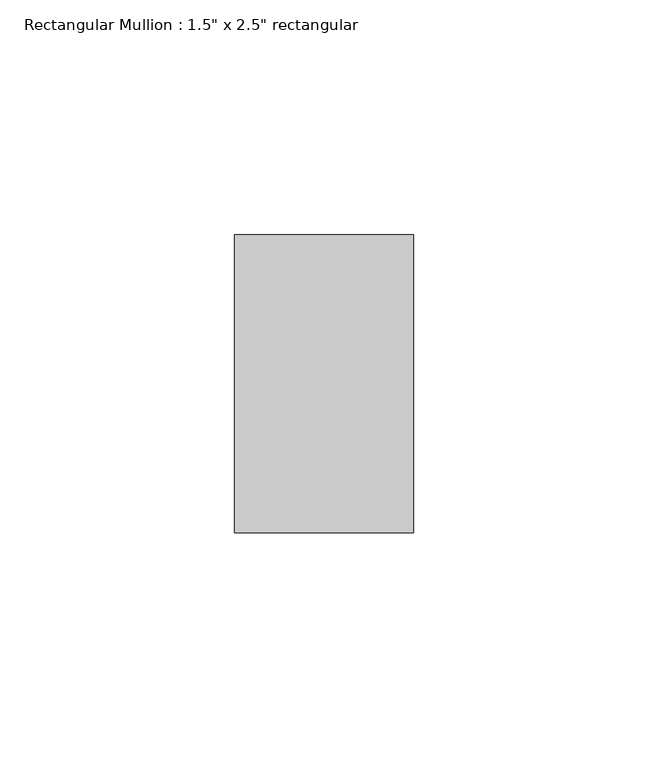
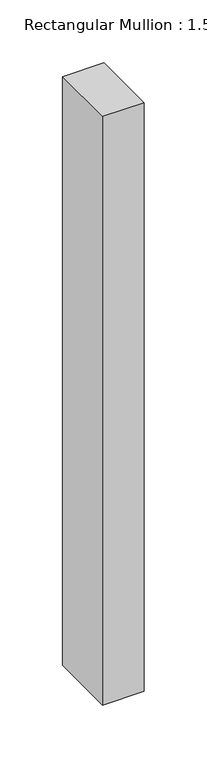
"""IFC4 building model written with IfcOpenShell, lengths in millimetres: member geometry."""

from ifc_helpers import new_model, si_unit, frame, origin, place, context, project, spatial, polyline, outline, extrude, source, transform, mapped, element, save


def member_b8e7570c(model_context):
    return source(origin(), model_context, "Body", "SweptSolid", [
        extrude(outline(polyline([(19.05, 31.75), (19.05, -31.75), (-19.05, -31.75), (-19.05, 31.75), (19.05, 31.75)])), frame((0.0, 0.0, -571.5), z_axis=(0.0, 0.0, 1.0), x_axis=(1.0, 0.0, 0.0)), (0.0, 0.0, 1.0), 571.5),
    ])


if __name__ == "__main__":
    model = new_model("IFC4")
    model_context = context("Model", 3, world=origin())
    ifc_project = project(units=[si_unit("LENGTHUNIT", "METRE", prefix="MILLI")], contexts=[model_context])
    site = spatial("IfcSite", under=ifc_project)
    building = spatial("IfcBuilding", under=site)
    placement = place(None, origin())
    member_shape = member_b8e7570c(model_context)
    element("IfcMember", 1, ObjectType="Rectangular Mullion : 1.5\" x 2.5\" rectangular", at=placement, inside=building, context=model_context, shape_type="MappedRepresentation", body=[
        mapped(member_shape, transform((0.0, 0.0, 0.0), x_axis=(1.0, 0.0, 0.0), y_axis=(0.0, 1.0, 0.0), z_axis=(0.0, 0.0, 1.0))),
    ])
    save(model, "model.ifc")

# Revit data of these elements
# Type "Rectangular Mullion : 1.5\" x 2.5\" rectangular"
#   built-in parameter 1007304 = 0.208333 (stored number, unit not read)
#   built-in parameter 1007301 = 0.0625 (stored number, unit not read)
#   built-in parameter 1007300 = 0.0625 (stored number, unit not read)
